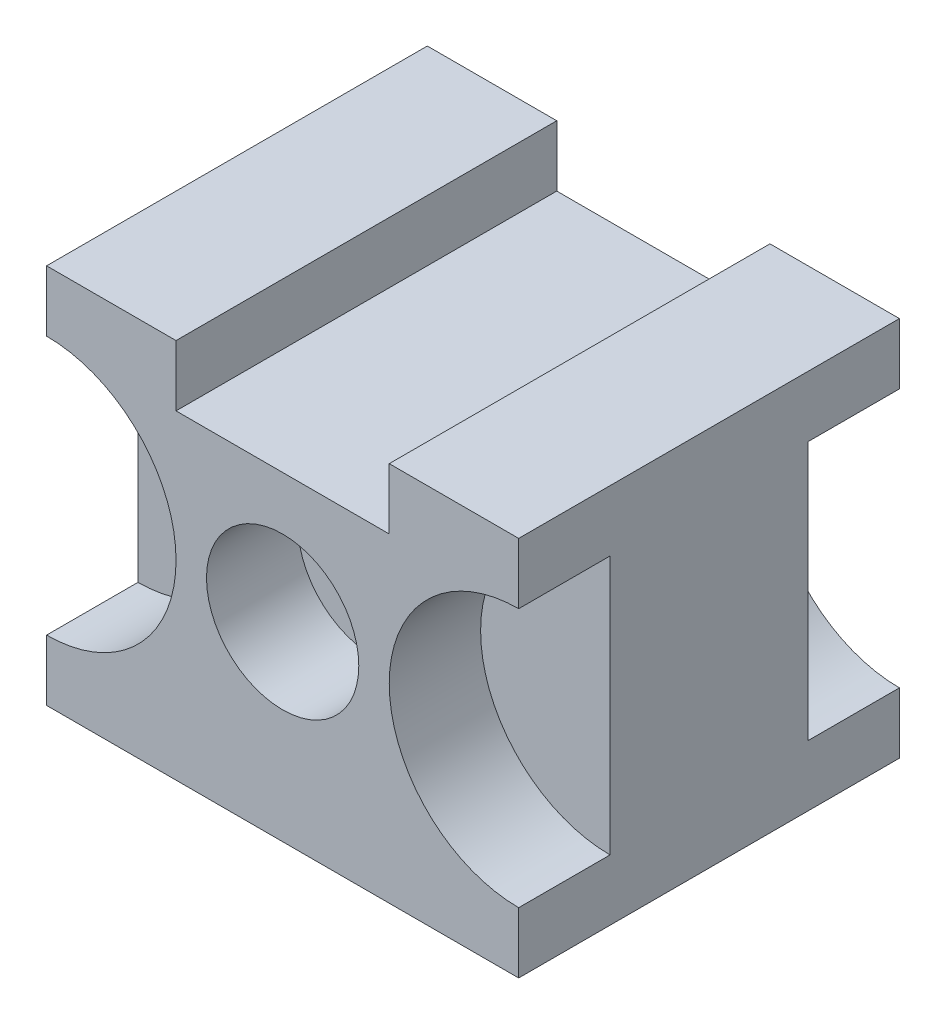
ISO-10303-21;
HEADER;
FILE_DESCRIPTION(('STEP AP214'),'2;1');
FILE_NAME('part.step','',(''),(''),'','','');
FILE_SCHEMA(('AUTOMOTIVE_DESIGN { 1 0 10303 214 1 1 1 1 }'));
ENDSEC;
DATA;
#1=APPLICATION_CONTEXT('core data for automotive mechanical design processes');
#2=APPLICATION_PROTOCOL_DEFINITION('international standard','automotive_design',2000,#1);
#3=PRODUCT_CONTEXT('',#1,'mechanical');
#4=PRODUCT('Part','Part','',(#3));
#5=PRODUCT_RELATED_PRODUCT_CATEGORY('part','',(#4));
#6=PRODUCT_DEFINITION_FORMATION('','',#4);
#7=PRODUCT_DEFINITION_CONTEXT('part definition',#1,'design');
#8=PRODUCT_DEFINITION('design','',#6,#7);
#9=PRODUCT_DEFINITION_SHAPE('','',#8);
#10=(LENGTH_UNIT() NAMED_UNIT(*) SI_UNIT(.MILLI.,.METRE.));
#11=(NAMED_UNIT(*) PLANE_ANGLE_UNIT() SI_UNIT($,.RADIAN.));
#12=(NAMED_UNIT(*) SI_UNIT($,.STERADIAN.) SOLID_ANGLE_UNIT());
#13=UNCERTAINTY_MEASURE_WITH_UNIT(LENGTH_MEASURE(1.E-05),#10,'distance_accuracy_value','');
#14=(GEOMETRIC_REPRESENTATION_CONTEXT(3) GLOBAL_UNCERTAINTY_ASSIGNED_CONTEXT((#13)) GLOBAL_UNIT_ASSIGNED_CONTEXT((#10,
#11,#12)) REPRESENTATION_CONTEXT('',''));
#15=CARTESIAN_POINT('',(0.,0.,0.));
#16=DIRECTION('',(0.,0.,1.));
#17=DIRECTION('',(1.,0.,0.));
#18=AXIS2_PLACEMENT_3D('',#15,#16,#17);
#19=CARTESIAN_POINT('',(62.,50.,50.));
#20=DIRECTION('',(0.,-1.,0.));
#21=DIRECTION('',(1.,0.,0.));
#22=AXIS2_PLACEMENT_3D('',#19,#20,#21);
#23=PLANE('',#22);
#24=DIRECTION('',(-1.,0.,0.));
#25=VECTOR('',#24,1.);
#26=CARTESIAN_POINT('',(62.,50.,50.));
#27=LINE('',#26,#25);
#28=CARTESIAN_POINT('',(17.,50.,50.));
#29=VERTEX_POINT('',#28);
#30=CARTESIAN_POINT('',(0.,50.,50.));
#31=VERTEX_POINT('',#30);
#32=EDGE_CURVE('E286',#29,#31,#27,.T.);
#33=ORIENTED_EDGE('',*,*,#32,.F.);
#34=DIRECTION('',(0.,0.,1.));
#35=VECTOR('',#34,1.);
#36=CARTESIAN_POINT('',(17.,50.,0.));
#37=LINE('',#36,#35);
#38=CARTESIAN_POINT('',(17.,50.,0.));
#39=VERTEX_POINT('',#38);
#40=EDGE_CURVE('E253',#39,#29,#37,.T.);
#41=ORIENTED_EDGE('',*,*,#40,.F.);
#42=DIRECTION('',(-1.,0.,0.));
#43=VECTOR('',#42,1.);
#44=CARTESIAN_POINT('',(62.,50.,0.));
#45=LINE('',#44,#43);
#46=CARTESIAN_POINT('',(0.,50.,0.));
#47=VERTEX_POINT('',#46);
#48=EDGE_CURVE('E299',#39,#47,#45,.T.);
#49=ORIENTED_EDGE('',*,*,#48,.T.);
#50=DIRECTION('',(0.,0.,-1.));
#51=VECTOR('',#50,1.);
#52=CARTESIAN_POINT('',(0.,50.,50.));
#53=LINE('',#52,#51);
#54=EDGE_CURVE('E295',#31,#47,#53,.T.);
#55=ORIENTED_EDGE('',*,*,#54,.F.);
#56=EDGE_LOOP('',(#33,#41,#49,#55));
#57=FACE_BOUND('',#56,.T.);
#58=ADVANCED_FACE('F39',(#57),#23,.F.);
#59=CARTESIAN_POINT('',(0.,50.,50.));
#60=DIRECTION('',(1.,0.,0.));
#61=DIRECTION('',(0.,1.,0.));
#62=AXIS2_PLACEMENT_3D('',#59,#60,#61);
#63=PLANE('',#62);
#64=DIRECTION('',(0.,0.,-1.));
#65=VECTOR('',#64,1.);
#66=CARTESIAN_POINT('',(0.,34.,25.));
#67=LINE('',#66,#65);
#68=CARTESIAN_POINT('',(0.,34.,32.));
#69=VERTEX_POINT('',#68);
#70=CARTESIAN_POINT('',(0.,34.,19.4759366020386));
#71=VERTEX_POINT('',#70);
#72=EDGE_CURVE('E199',#69,#71,#67,.T.);
#73=ORIENTED_EDGE('',*,*,#72,.F.);
#74=DIRECTION('',(0.,1.,0.));
#75=VECTOR('',#74,1.);
#76=CARTESIAN_POINT('',(0.,16.,32.));
#77=LINE('',#76,#75);
#78=CARTESIAN_POINT('',(0.,16.,32.));
#79=VERTEX_POINT('',#78);
#80=EDGE_CURVE('E204',#79,#69,#77,.T.);
#81=ORIENTED_EDGE('',*,*,#80,.F.);
#82=DIRECTION('',(0.,0.,1.));
#83=VECTOR('',#82,1.);
#84=CARTESIAN_POINT('',(0.,16.,19.4759366020386));
#85=LINE('',#84,#83);
#86=CARTESIAN_POINT('',(0.,16.,19.4759366020386));
#87=VERTEX_POINT('',#86);
#88=EDGE_CURVE('E218',#87,#79,#85,.T.);
#89=ORIENTED_EDGE('',*,*,#88,.F.);
#90=DIRECTION('',(0.,-1.,0.));
#91=VECTOR('',#90,1.);
#92=CARTESIAN_POINT('',(0.,34.,19.4759366020386));
#93=LINE('',#92,#91);
#94=EDGE_CURVE('E216',#71,#87,#93,.T.);
#95=ORIENTED_EDGE('',*,*,#94,.F.);
#96=EDGE_LOOP('',(#73,#81,#89,#95));
#97=FACE_BOUND('',#96,.T.);
#98=DIRECTION('',(0.,1.,0.));
#99=VECTOR('',#98,1.);
#100=CARTESIAN_POINT('',(0.,50.,12.));
#101=LINE('',#100,#99);
#102=CARTESIAN_POINT('',(0.,8.,12.));
#103=VERTEX_POINT('',#102);
#104=CARTESIAN_POINT('',(0.,42.,12.));
#105=VERTEX_POINT('',#104);
#106=EDGE_CURVE('E11',#103,#105,#101,.T.);
#107=ORIENTED_EDGE('',*,*,#106,.F.);
#108=DIRECTION('',(0.,0.,-1.));
#109=VECTOR('',#108,1.);
#110=CARTESIAN_POINT('',(0.,8.00000000000001,12.));
#111=LINE('',#110,#109);
#112=CARTESIAN_POINT('',(0.,8.,0.));
#113=VERTEX_POINT('',#112);
#114=EDGE_CURVE('E185',#103,#113,#111,.T.);
#115=ORIENTED_EDGE('',*,*,#114,.T.);
#116=DIRECTION('',(0.,-1.,0.));
#117=VECTOR('',#116,1.);
#118=CARTESIAN_POINT('',(0.,50.,0.));
#119=LINE('',#118,#117);
#120=CARTESIAN_POINT('',(0.,0.,0.));
#121=VERTEX_POINT('',#120);
#122=EDGE_CURVE('E280',#113,#121,#119,.T.);
#123=ORIENTED_EDGE('',*,*,#122,.T.);
#124=DIRECTION('',(0.,0.,-1.));
#125=VECTOR('',#124,1.);
#126=CARTESIAN_POINT('',(0.,0.,50.));
#127=LINE('',#126,#125);
#128=CARTESIAN_POINT('',(0.,0.,50.));
#129=VERTEX_POINT('',#128);
#130=EDGE_CURVE('E313',#129,#121,#127,.T.);
#131=ORIENTED_EDGE('',*,*,#130,.F.);
#132=DIRECTION('',(0.,-1.,0.));
#133=VECTOR('',#132,1.);
#134=CARTESIAN_POINT('',(0.,50.,50.));
#135=LINE('',#134,#133);
#136=CARTESIAN_POINT('',(0.,8.00000000000001,50.));
#137=VERTEX_POINT('',#136);
#138=EDGE_CURVE('E285',#137,#129,#135,.T.);
#139=ORIENTED_EDGE('',*,*,#138,.F.);
#140=DIRECTION('',(0.,0.,1.));
#141=VECTOR('',#140,1.);
#142=CARTESIAN_POINT('',(0.,8.00000000000001,38.));
#143=LINE('',#142,#141);
#144=CARTESIAN_POINT('',(0.,8.,38.));
#145=VERTEX_POINT('',#144);
#146=EDGE_CURVE('E261',#137,#145,#143,.F.);
#147=ORIENTED_EDGE('',*,*,#146,.T.);
#148=DIRECTION('',(0.,-1.,0.));
#149=VECTOR('',#148,1.);
#150=CARTESIAN_POINT('',(0.,50.,38.));
#151=LINE('',#150,#149);
#152=CARTESIAN_POINT('',(0.,42.,38.));
#153=VERTEX_POINT('',#152);
#154=EDGE_CURVE('E318',#153,#145,#151,.T.);
#155=ORIENTED_EDGE('',*,*,#154,.F.);
#156=DIRECTION('',(0.,0.,1.));
#157=VECTOR('',#156,1.);
#158=CARTESIAN_POINT('',(0.,42.,38.));
#159=LINE('',#158,#157);
#160=CARTESIAN_POINT('',(0.,42.,50.));
#161=VERTEX_POINT('',#160);
#162=EDGE_CURVE('E268',#153,#161,#159,.T.);
#163=ORIENTED_EDGE('',*,*,#162,.T.);
#164=EDGE_CURVE('E279',#31,#161,#135,.T.);
#165=ORIENTED_EDGE('',*,*,#164,.F.);
#166=ORIENTED_EDGE('',*,*,#54,.T.);
#167=CARTESIAN_POINT('',(0.,42.,0.));
#168=VERTEX_POINT('',#167);
#169=EDGE_CURVE('E188',#47,#168,#119,.T.);
#170=ORIENTED_EDGE('',*,*,#169,.T.);
#171=DIRECTION('',(0.,0.,-1.));
#172=VECTOR('',#171,1.);
#173=CARTESIAN_POINT('',(0.,42.,12.));
#174=LINE('',#173,#172);
#175=EDGE_CURVE('E53',#168,#105,#174,.F.);
#176=ORIENTED_EDGE('',*,*,#175,.T.);
#177=EDGE_LOOP('',(#107,#115,#123,#131,#139,#147,#155,#163,#165,#166,#170,#176));
#178=FACE_BOUND('',#177,.T.);
#179=ADVANCED_FACE('F41',(#97,#178),#63,.F.);
#180=CARTESIAN_POINT('',(0.,0.,50.));
#181=DIRECTION('',(0.,1.,0.));
#182=DIRECTION('',(0.,0.,1.));
#183=AXIS2_PLACEMENT_3D('',#180,#181,#182);
#184=PLANE('',#183);
#185=DIRECTION('',(1.,0.,0.));
#186=VECTOR('',#185,1.);
#187=CARTESIAN_POINT('',(0.,0.,0.));
#188=LINE('',#187,#186);
#189=CARTESIAN_POINT('',(62.,0.,0.));
#190=VERTEX_POINT('',#189);
#191=EDGE_CURVE('E294',#121,#190,#188,.T.);
#192=ORIENTED_EDGE('',*,*,#191,.T.);
#193=DIRECTION('',(0.,0.,-1.));
#194=VECTOR('',#193,1.);
#195=CARTESIAN_POINT('',(62.,0.,50.));
#196=LINE('',#195,#194);
#197=CARTESIAN_POINT('',(62.,0.,50.));
#198=VERTEX_POINT('',#197);
#199=EDGE_CURVE('E306',#198,#190,#196,.T.);
#200=ORIENTED_EDGE('',*,*,#199,.F.);
#201=DIRECTION('',(1.,0.,0.));
#202=VECTOR('',#201,1.);
#203=CARTESIAN_POINT('',(0.,0.,50.));
#204=LINE('',#203,#202);
#205=EDGE_CURVE('E281',#129,#198,#204,.T.);
#206=ORIENTED_EDGE('',*,*,#205,.F.);
#207=ORIENTED_EDGE('',*,*,#130,.T.);
#208=EDGE_LOOP('',(#192,#200,#206,#207));
#209=FACE_BOUND('',#208,.T.);
#210=ADVANCED_FACE('F376',(#209),#184,.F.);
#211=CARTESIAN_POINT('',(62.,0.,50.));
#212=DIRECTION('',(-1.,0.,0.));
#213=DIRECTION('',(0.,0.,1.));
#214=AXIS2_PLACEMENT_3D('',#211,#212,#213);
#215=PLANE('',#214);
#216=DIRECTION('',(0.,-1.,0.));
#217=VECTOR('',#216,1.);
#218=CARTESIAN_POINT('',(62.,0.,12.));
#219=LINE('',#218,#217);
#220=CARTESIAN_POINT('',(62.,42.,12.));
#221=VERTEX_POINT('',#220);
#222=CARTESIAN_POINT('',(62.,8.,12.));
#223=VERTEX_POINT('',#222);
#224=EDGE_CURVE('E50',#221,#223,#219,.T.);
#225=ORIENTED_EDGE('',*,*,#224,.F.);
#226=DIRECTION('',(0.,0.,-1.));
#227=VECTOR('',#226,1.);
#228=CARTESIAN_POINT('',(62.,42.,12.));
#229=LINE('',#228,#227);
#230=CARTESIAN_POINT('',(62.,42.,0.));
#231=VERTEX_POINT('',#230);
#232=EDGE_CURVE('E197',#221,#231,#229,.T.);
#233=ORIENTED_EDGE('',*,*,#232,.T.);
#234=DIRECTION('',(0.,1.,0.));
#235=VECTOR('',#234,1.);
#236=CARTESIAN_POINT('',(62.,0.,0.));
#237=LINE('',#236,#235);
#238=CARTESIAN_POINT('',(62.,50.,0.));
#239=VERTEX_POINT('',#238);
#240=EDGE_CURVE('E296',#231,#239,#237,.T.);
#241=ORIENTED_EDGE('',*,*,#240,.T.);
#242=DIRECTION('',(0.,0.,-1.));
#243=VECTOR('',#242,1.);
#244=CARTESIAN_POINT('',(62.,50.,50.));
#245=LINE('',#244,#243);
#246=CARTESIAN_POINT('',(62.,50.,50.));
#247=VERTEX_POINT('',#246);
#248=EDGE_CURVE('E304',#247,#239,#245,.T.);
#249=ORIENTED_EDGE('',*,*,#248,.F.);
#250=DIRECTION('',(0.,1.,0.));
#251=VECTOR('',#250,1.);
#252=CARTESIAN_POINT('',(62.,0.,50.));
#253=LINE('',#252,#251);
#254=CARTESIAN_POINT('',(62.,42.,50.));
#255=VERTEX_POINT('',#254);
#256=EDGE_CURVE('E283',#255,#247,#253,.T.);
#257=ORIENTED_EDGE('',*,*,#256,.F.);
#258=DIRECTION('',(0.,0.,1.));
#259=VECTOR('',#258,1.);
#260=CARTESIAN_POINT('',(62.,42.,38.));
#261=LINE('',#260,#259);
#262=CARTESIAN_POINT('',(62.,42.,38.));
#263=VERTEX_POINT('',#262);
#264=EDGE_CURVE('E271',#255,#263,#261,.F.);
#265=ORIENTED_EDGE('',*,*,#264,.T.);
#266=DIRECTION('',(0.,1.,0.));
#267=VECTOR('',#266,1.);
#268=CARTESIAN_POINT('',(62.,0.,38.));
#269=LINE('',#268,#267);
#270=CARTESIAN_POINT('',(62.,8.00000000000001,38.));
#271=VERTEX_POINT('',#270);
#272=EDGE_CURVE('E316',#271,#263,#269,.T.);
#273=ORIENTED_EDGE('',*,*,#272,.F.);
#274=DIRECTION('',(0.,0.,1.));
#275=VECTOR('',#274,1.);
#276=CARTESIAN_POINT('',(62.,8.00000000000001,38.));
#277=LINE('',#276,#275);
#278=CARTESIAN_POINT('',(62.,8.00000000000001,50.));
#279=VERTEX_POINT('',#278);
#280=EDGE_CURVE('E273',#271,#279,#277,.T.);
#281=ORIENTED_EDGE('',*,*,#280,.T.);
#282=EDGE_CURVE('E284',#198,#279,#253,.T.);
#283=ORIENTED_EDGE('',*,*,#282,.F.);
#284=ORIENTED_EDGE('',*,*,#199,.T.);
#285=CARTESIAN_POINT('',(62.,8.,0.));
#286=VERTEX_POINT('',#285);
#287=EDGE_CURVE('E300',#190,#286,#237,.T.);
#288=ORIENTED_EDGE('',*,*,#287,.T.);
#289=DIRECTION('',(0.,0.,-1.));
#290=VECTOR('',#289,1.);
#291=CARTESIAN_POINT('',(62.,8.,12.));
#292=LINE('',#291,#290);
#293=EDGE_CURVE('E65',#286,#223,#292,.F.);
#294=ORIENTED_EDGE('',*,*,#293,.T.);
#295=EDGE_LOOP('',(#225,#233,#241,#249,#257,#265,#273,#281,#283,#284,#288,#294));
#296=FACE_BOUND('',#295,.T.);
#297=ADVANCED_FACE('F326',(#296),#215,.F.);
#298=CARTESIAN_POINT('',(45.,50.,0.));
#299=VERTEX_POINT('',#298);
#300=EDGE_CURVE('E303',#239,#299,#45,.T.);
#301=ORIENTED_EDGE('',*,*,#300,.T.);
#302=DIRECTION('',(0.,0.,1.));
#303=VECTOR('',#302,1.);
#304=CARTESIAN_POINT('',(45.,50.,0.));
#305=LINE('',#304,#303);
#306=CARTESIAN_POINT('',(45.,50.,50.));
#307=VERTEX_POINT('',#306);
#308=EDGE_CURVE('E251',#299,#307,#305,.T.);
#309=ORIENTED_EDGE('',*,*,#308,.T.);
#310=EDGE_CURVE('E287',#247,#307,#27,.T.);
#311=ORIENTED_EDGE('',*,*,#310,.F.);
#312=ORIENTED_EDGE('',*,*,#248,.T.);
#313=EDGE_LOOP('',(#301,#309,#311,#312));
#314=FACE_BOUND('',#313,.T.);
#315=ADVANCED_FACE('F339',(#314),#23,.F.);
#316=CARTESIAN_POINT('',(0.,0.,50.));
#317=DIRECTION('',(0.,0.,1.));
#318=DIRECTION('',(1.,0.,0.));
#319=AXIS2_PLACEMENT_3D('',#316,#317,#318);
#320=PLANE('',#319);
#321=CARTESIAN_POINT('',(31.,25.,50.));
#322=DIRECTION('',(0.,0.,1.));
#323=DIRECTION('',(1.,0.,0.));
#324=AXIS2_PLACEMENT_3D('',#321,#322,#323);
#325=CIRCLE('',#324,10.);
#326=CARTESIAN_POINT('',(41.,25.,50.));
#327=VERTEX_POINT('',#326);
#328=EDGE_CURVE('E405',#327,#327,#325,.T.);
#329=ORIENTED_EDGE('',*,*,#328,.F.);
#330=EDGE_LOOP('',(#329));
#331=FACE_BOUND('',#330,.T.);
#332=DIRECTION('',(0.,-1.,0.));
#333=VECTOR('',#332,1.);
#334=CARTESIAN_POINT('',(17.,42.,50.));
#335=LINE('',#334,#333);
#336=CARTESIAN_POINT('',(17.,42.,50.));
#337=VERTEX_POINT('',#336);
#338=EDGE_CURVE('E243',#29,#337,#335,.T.);
#339=ORIENTED_EDGE('',*,*,#338,.F.);
#340=ORIENTED_EDGE('',*,*,#32,.T.);
#341=ORIENTED_EDGE('',*,*,#164,.T.);
#342=CARTESIAN_POINT('',(0.,25.,50.));
#343=DIRECTION('',(0.,0.,1.));
#344=DIRECTION('',(1.,0.,0.));
#345=AXIS2_PLACEMENT_3D('',#342,#343,#344);
#346=CIRCLE('',#345,17.);
#347=EDGE_CURVE('E314',#137,#161,#346,.T.);
#348=ORIENTED_EDGE('',*,*,#347,.F.);
#349=ORIENTED_EDGE('',*,*,#138,.T.);
#350=ORIENTED_EDGE('',*,*,#205,.T.);
#351=ORIENTED_EDGE('',*,*,#282,.T.);
#352=CARTESIAN_POINT('',(62.,25.,50.));
#353=DIRECTION('',(0.,0.,1.));
#354=DIRECTION('',(1.,0.,0.));
#355=AXIS2_PLACEMENT_3D('',#352,#353,#354);
#356=CIRCLE('',#355,17.);
#357=EDGE_CURVE('E265',#255,#279,#356,.T.);
#358=ORIENTED_EDGE('',*,*,#357,.F.);
#359=ORIENTED_EDGE('',*,*,#256,.T.);
#360=ORIENTED_EDGE('',*,*,#310,.T.);
#361=DIRECTION('',(0.,1.,0.));
#362=VECTOR('',#361,1.);
#363=CARTESIAN_POINT('',(45.,50.,50.));
#364=LINE('',#363,#362);
#365=CARTESIAN_POINT('',(45.,42.,50.));
#366=VERTEX_POINT('',#365);
#367=EDGE_CURVE('E226',#366,#307,#364,.T.);
#368=ORIENTED_EDGE('',*,*,#367,.F.);
#369=DIRECTION('',(1.,0.,0.));
#370=VECTOR('',#369,1.);
#371=CARTESIAN_POINT('',(31.,42.,50.));
#372=LINE('',#371,#370);
#373=EDGE_CURVE('E237',#337,#366,#372,.T.);
#374=ORIENTED_EDGE('',*,*,#373,.F.);
#375=EDGE_LOOP('',(#339,#340,#341,#348,#349,#350,#351,#358,#359,#360,#368,#374));
#376=FACE_BOUND('',#375,.T.);
#377=ADVANCED_FACE('F350',(#331,#376),#320,.T.);
#378=CARTESIAN_POINT('',(0.,0.,0.));
#379=DIRECTION('',(0.,0.,1.));
#380=DIRECTION('',(1.,0.,0.));
#381=AXIS2_PLACEMENT_3D('',#378,#379,#380);
#382=PLANE('',#381);
#383=ORIENTED_EDGE('',*,*,#240,.F.);
#384=CARTESIAN_POINT('',(62.,25.,0.));
#385=DIRECTION('',(0.,0.,1.));
#386=DIRECTION('',(1.,0.,0.));
#387=AXIS2_PLACEMENT_3D('',#384,#385,#386);
#388=CIRCLE('',#387,17.);
#389=EDGE_CURVE('E319',#231,#286,#388,.T.);
#390=ORIENTED_EDGE('',*,*,#389,.T.);
#391=ORIENTED_EDGE('',*,*,#287,.F.);
#392=ORIENTED_EDGE('',*,*,#191,.F.);
#393=ORIENTED_EDGE('',*,*,#122,.F.);
#394=CARTESIAN_POINT('',(0.,25.,0.));
#395=DIRECTION('',(0.,0.,-1.));
#396=DIRECTION('',(-1.,0.,0.));
#397=AXIS2_PLACEMENT_3D('',#394,#395,#396);
#398=CIRCLE('',#397,17.);
#399=EDGE_CURVE('E184',#168,#113,#398,.T.);
#400=ORIENTED_EDGE('',*,*,#399,.F.);
#401=ORIENTED_EDGE('',*,*,#169,.F.);
#402=ORIENTED_EDGE('',*,*,#48,.F.);
#403=DIRECTION('',(0.,-1.,0.));
#404=VECTOR('',#403,1.);
#405=CARTESIAN_POINT('',(17.,42.,0.));
#406=LINE('',#405,#404);
#407=CARTESIAN_POINT('',(17.,42.,0.));
#408=VERTEX_POINT('',#407);
#409=EDGE_CURVE('E239',#39,#408,#406,.T.);
#410=ORIENTED_EDGE('',*,*,#409,.T.);
#411=DIRECTION('',(1.,0.,0.));
#412=VECTOR('',#411,1.);
#413=CARTESIAN_POINT('',(45.,42.,0.));
#414=LINE('',#413,#412);
#415=CARTESIAN_POINT('',(45.,42.,0.));
#416=VERTEX_POINT('',#415);
#417=EDGE_CURVE('E235',#408,#416,#414,.T.);
#418=ORIENTED_EDGE('',*,*,#417,.T.);
#419=DIRECTION('',(0.,1.,0.));
#420=VECTOR('',#419,1.);
#421=CARTESIAN_POINT('',(45.,50.,0.));
#422=LINE('',#421,#420);
#423=EDGE_CURVE('E234',#416,#299,#422,.T.);
#424=ORIENTED_EDGE('',*,*,#423,.T.);
#425=ORIENTED_EDGE('',*,*,#300,.F.);
#426=EDGE_LOOP('',(#383,#390,#391,#392,#393,#400,#401,#402,#410,#418,#424,#425));
#427=FACE_BOUND('',#426,.T.);
#428=ADVANCED_FACE('F334',(#427),#382,.F.);
#429=CARTESIAN_POINT('',(0.,25.,38.));
#430=DIRECTION('',(0.,0.,1.));
#431=DIRECTION('',(1.,0.,0.));
#432=AXIS2_PLACEMENT_3D('',#429,#430,#431);
#433=PLANE('',#432);
#434=ORIENTED_EDGE('',*,*,#154,.T.);
#435=CARTESIAN_POINT('',(0.,25.,38.));
#436=DIRECTION('',(0.,0.,1.));
#437=DIRECTION('',(1.,0.,0.));
#438=AXIS2_PLACEMENT_3D('',#435,#436,#437);
#439=CIRCLE('',#438,17.);
#440=EDGE_CURVE('E249',#145,#153,#439,.T.);
#441=ORIENTED_EDGE('',*,*,#440,.T.);
#442=EDGE_LOOP('',(#434,#441));
#443=FACE_BOUND('',#442,.T.);
#444=ADVANCED_FACE('F364',(#443),#433,.T.);
#445=CARTESIAN_POINT('',(0.,25.,38.));
#446=DIRECTION('',(0.,0.,1.));
#447=DIRECTION('',(1.,0.,0.));
#448=AXIS2_PLACEMENT_3D('',#445,#446,#447);
#449=CYLINDRICAL_SURFACE('',#448,17.);
#450=ORIENTED_EDGE('',*,*,#440,.F.);
#451=ORIENTED_EDGE('',*,*,#146,.F.);
#452=ORIENTED_EDGE('',*,*,#347,.T.);
#453=ORIENTED_EDGE('',*,*,#162,.F.);
#454=EDGE_LOOP('',(#450,#451,#452,#453));
#455=FACE_BOUND('',#454,.T.);
#456=ADVANCED_FACE('F360',(#455),#449,.F.);
#457=CARTESIAN_POINT('',(62.,25.,38.));
#458=DIRECTION('',(0.,0.,1.));
#459=DIRECTION('',(1.,0.,0.));
#460=AXIS2_PLACEMENT_3D('',#457,#458,#459);
#461=PLANE('',#460);
#462=ORIENTED_EDGE('',*,*,#272,.T.);
#463=CARTESIAN_POINT('',(62.,25.,38.));
#464=DIRECTION('',(0.,0.,1.));
#465=DIRECTION('',(1.,0.,0.));
#466=AXIS2_PLACEMENT_3D('',#463,#464,#465);
#467=CIRCLE('',#466,17.);
#468=EDGE_CURVE('E256',#263,#271,#467,.T.);
#469=ORIENTED_EDGE('',*,*,#468,.T.);
#470=EDGE_LOOP('',(#462,#469));
#471=FACE_BOUND('',#470,.T.);
#472=ADVANCED_FACE('F354',(#471),#461,.T.);
#473=CARTESIAN_POINT('',(62.,25.,38.));
#474=DIRECTION('',(0.,0.,1.));
#475=DIRECTION('',(1.,0.,0.));
#476=AXIS2_PLACEMENT_3D('',#473,#474,#475);
#477=CYLINDRICAL_SURFACE('',#476,17.);
#478=ORIENTED_EDGE('',*,*,#468,.F.);
#479=ORIENTED_EDGE('',*,*,#264,.F.);
#480=ORIENTED_EDGE('',*,*,#357,.T.);
#481=ORIENTED_EDGE('',*,*,#280,.F.);
#482=EDGE_LOOP('',(#478,#479,#480,#481));
#483=FACE_BOUND('',#482,.T.);
#484=ADVANCED_FACE('F352',(#483),#477,.F.);
#485=CARTESIAN_POINT('',(31.,42.,0.));
#486=DIRECTION('',(0.,-1.,0.));
#487=DIRECTION('',(1.,0.,0.));
#488=AXIS2_PLACEMENT_3D('',#485,#486,#487);
#489=PLANE('',#488);
#490=ORIENTED_EDGE('',*,*,#373,.T.);
#491=DIRECTION('',(0.,0.,1.));
#492=VECTOR('',#491,1.);
#493=CARTESIAN_POINT('',(45.,42.,0.));
#494=LINE('',#493,#492);
#495=EDGE_CURVE('E245',#416,#366,#494,.T.);
#496=ORIENTED_EDGE('',*,*,#495,.F.);
#497=ORIENTED_EDGE('',*,*,#417,.F.);
#498=DIRECTION('',(0.,0.,1.));
#499=VECTOR('',#498,1.);
#500=CARTESIAN_POINT('',(17.,42.,0.));
#501=LINE('',#500,#499);
#502=EDGE_CURVE('E246',#408,#337,#501,.T.);
#503=ORIENTED_EDGE('',*,*,#502,.T.);
#504=EDGE_LOOP('',(#490,#496,#497,#503));
#505=FACE_BOUND('',#504,.T.);
#506=ADVANCED_FACE('F361',(#505),#489,.F.);
#507=CARTESIAN_POINT('',(17.,42.,0.));
#508=DIRECTION('',(-1.,0.,0.));
#509=DIRECTION('',(0.,0.,1.));
#510=AXIS2_PLACEMENT_3D('',#507,#508,#509);
#511=PLANE('',#510);
#512=ORIENTED_EDGE('',*,*,#338,.T.);
#513=ORIENTED_EDGE('',*,*,#502,.F.);
#514=ORIENTED_EDGE('',*,*,#409,.F.);
#515=ORIENTED_EDGE('',*,*,#40,.T.);
#516=EDGE_LOOP('',(#512,#513,#514,#515));
#517=FACE_BOUND('',#516,.T.);
#518=ADVANCED_FACE('F448',(#517),#511,.F.);
#519=CARTESIAN_POINT('',(45.,50.,0.));
#520=DIRECTION('',(1.,0.,0.));
#521=DIRECTION('',(0.,0.,-1.));
#522=AXIS2_PLACEMENT_3D('',#519,#520,#521);
#523=PLANE('',#522);
#524=ORIENTED_EDGE('',*,*,#367,.T.);
#525=ORIENTED_EDGE('',*,*,#308,.F.);
#526=ORIENTED_EDGE('',*,*,#423,.F.);
#527=ORIENTED_EDGE('',*,*,#495,.T.);
#528=EDGE_LOOP('',(#524,#525,#526,#527));
#529=FACE_BOUND('',#528,.T.);
#530=ADVANCED_FACE('F341',(#529),#523,.F.);
#531=CARTESIAN_POINT('',(12.,16.,32.));
#532=DIRECTION('',(0.,0.,1.));
#533=DIRECTION('',(0.,-1.,0.));
#534=AXIS2_PLACEMENT_3D('',#531,#532,#533);
#535=PLANE('',#534);
#536=ORIENTED_EDGE('',*,*,#80,.T.);
#537=DIRECTION('',(-1.,0.,0.));
#538=VECTOR('',#537,1.);
#539=CARTESIAN_POINT('',(12.,34.,32.));
#540=LINE('',#539,#538);
#541=CARTESIAN_POINT('',(12.,34.,32.));
#542=VERTEX_POINT('',#541);
#543=EDGE_CURVE('E224',#542,#69,#540,.T.);
#544=ORIENTED_EDGE('',*,*,#543,.F.);
#545=DIRECTION('',(0.,1.,0.));
#546=VECTOR('',#545,1.);
#547=CARTESIAN_POINT('',(12.,16.,32.));
#548=LINE('',#547,#546);
#549=CARTESIAN_POINT('',(12.,16.,32.));
#550=VERTEX_POINT('',#549);
#551=EDGE_CURVE('E209',#550,#542,#548,.T.);
#552=ORIENTED_EDGE('',*,*,#551,.F.);
#553=DIRECTION('',(-1.,0.,0.));
#554=VECTOR('',#553,1.);
#555=CARTESIAN_POINT('',(12.,16.,32.));
#556=LINE('',#555,#554);
#557=EDGE_CURVE('E230',#550,#79,#556,.T.);
#558=ORIENTED_EDGE('',*,*,#557,.T.);
#559=EDGE_LOOP('',(#536,#544,#552,#558));
#560=FACE_BOUND('',#559,.T.);
#561=ADVANCED_FACE('F433',(#560),#535,.F.);
#562=CARTESIAN_POINT('',(12.,16.,19.4759366020386));
#563=DIRECTION('',(0.,-1.,0.));
#564=DIRECTION('',(1.,0.,0.));
#565=AXIS2_PLACEMENT_3D('',#562,#563,#564);
#566=PLANE('',#565);
#567=ORIENTED_EDGE('',*,*,#88,.T.);
#568=ORIENTED_EDGE('',*,*,#557,.F.);
#569=DIRECTION('',(0.,0.,1.));
#570=VECTOR('',#569,1.);
#571=CARTESIAN_POINT('',(12.,16.,19.4759366020386));
#572=LINE('',#571,#570);
#573=CARTESIAN_POINT('',(12.,16.,19.4759366020386));
#574=VERTEX_POINT('',#573);
#575=EDGE_CURVE('E210',#574,#550,#572,.T.);
#576=ORIENTED_EDGE('',*,*,#575,.F.);
#577=DIRECTION('',(-1.,0.,0.));
#578=VECTOR('',#577,1.);
#579=CARTESIAN_POINT('',(12.,16.,19.4759366020386));
#580=LINE('',#579,#578);
#581=EDGE_CURVE('E228',#574,#87,#580,.T.);
#582=ORIENTED_EDGE('',*,*,#581,.T.);
#583=EDGE_LOOP('',(#567,#568,#576,#582));
#584=FACE_BOUND('',#583,.T.);
#585=ADVANCED_FACE('F436',(#584),#566,.F.);
#586=CARTESIAN_POINT('',(12.,34.,19.4759366020386));
#587=DIRECTION('',(0.,0.,-1.));
#588=DIRECTION('',(0.,1.,0.));
#589=AXIS2_PLACEMENT_3D('',#586,#587,#588);
#590=PLANE('',#589);
#591=ORIENTED_EDGE('',*,*,#94,.T.);
#592=ORIENTED_EDGE('',*,*,#581,.F.);
#593=DIRECTION('',(0.,-1.,0.));
#594=VECTOR('',#593,1.);
#595=CARTESIAN_POINT('',(12.,34.,19.4759366020386));
#596=LINE('',#595,#594);
#597=CARTESIAN_POINT('',(12.,34.,19.4759366020386));
#598=VERTEX_POINT('',#597);
#599=EDGE_CURVE('E201',#598,#574,#596,.T.);
#600=ORIENTED_EDGE('',*,*,#599,.F.);
#601=DIRECTION('',(-1.,0.,0.));
#602=VECTOR('',#601,1.);
#603=CARTESIAN_POINT('',(12.,34.,19.4759366020386));
#604=LINE('',#603,#602);
#605=EDGE_CURVE('E213',#598,#71,#604,.T.);
#606=ORIENTED_EDGE('',*,*,#605,.T.);
#607=EDGE_LOOP('',(#591,#592,#600,#606));
#608=FACE_BOUND('',#607,.T.);
#609=ADVANCED_FACE('F439',(#608),#590,.F.);
#610=CARTESIAN_POINT('',(12.,34.,25.));
#611=DIRECTION('',(0.,1.,0.));
#612=DIRECTION('',(-1.,0.,0.));
#613=AXIS2_PLACEMENT_3D('',#610,#611,#612);
#614=PLANE('',#613);
#615=ORIENTED_EDGE('',*,*,#72,.T.);
#616=ORIENTED_EDGE('',*,*,#605,.F.);
#617=DIRECTION('',(0.,0.,-1.));
#618=VECTOR('',#617,1.);
#619=CARTESIAN_POINT('',(12.,34.,32.));
#620=LINE('',#619,#618);
#621=EDGE_CURVE('E203',#542,#598,#620,.T.);
#622=ORIENTED_EDGE('',*,*,#621,.F.);
#623=ORIENTED_EDGE('',*,*,#543,.T.);
#624=EDGE_LOOP('',(#615,#616,#622,#623));
#625=FACE_BOUND('',#624,.T.);
#626=ADVANCED_FACE('F431',(#625),#614,.F.);
#627=CARTESIAN_POINT('',(12.,0.,0.));
#628=DIRECTION('',(-1.,0.,0.));
#629=DIRECTION('',(0.,-1.,0.));
#630=AXIS2_PLACEMENT_3D('',#627,#628,#629);
#631=PLANE('',#630);
#632=ORIENTED_EDGE('',*,*,#621,.T.);
#633=ORIENTED_EDGE('',*,*,#599,.T.);
#634=ORIENTED_EDGE('',*,*,#575,.T.);
#635=ORIENTED_EDGE('',*,*,#551,.T.);
#636=EDGE_LOOP('',(#632,#633,#634,#635));
#637=FACE_BOUND('',#636,.T.);
#638=ADVANCED_FACE('F426',(#637),#631,.T.);
#639=CARTESIAN_POINT('',(0.,25.,12.));
#640=DIRECTION('',(0.,0.,-1.));
#641=DIRECTION('',(-1.,0.,0.));
#642=AXIS2_PLACEMENT_3D('',#639,#640,#641);
#643=PLANE('',#642);
#644=ORIENTED_EDGE('',*,*,#106,.T.);
#645=CARTESIAN_POINT('',(0.,25.,12.));
#646=DIRECTION('',(0.,0.,-1.));
#647=DIRECTION('',(-1.,0.,0.));
#648=AXIS2_PLACEMENT_3D('',#645,#646,#647);
#649=CIRCLE('',#648,17.);
#650=EDGE_CURVE('E176',#105,#103,#649,.T.);
#651=ORIENTED_EDGE('',*,*,#650,.T.);
#652=EDGE_LOOP('',(#644,#651));
#653=FACE_BOUND('',#652,.T.);
#654=ADVANCED_FACE('F180',(#653),#643,.T.);
#655=CARTESIAN_POINT('',(0.,25.,12.));
#656=DIRECTION('',(0.,0.,-1.));
#657=DIRECTION('',(-1.,0.,0.));
#658=AXIS2_PLACEMENT_3D('',#655,#656,#657);
#659=CYLINDRICAL_SURFACE('',#658,17.);
#660=ORIENTED_EDGE('',*,*,#650,.F.);
#661=ORIENTED_EDGE('',*,*,#175,.F.);
#662=ORIENTED_EDGE('',*,*,#399,.T.);
#663=ORIENTED_EDGE('',*,*,#114,.F.);
#664=EDGE_LOOP('',(#660,#661,#662,#663));
#665=FACE_BOUND('',#664,.T.);
#666=ADVANCED_FACE('F182',(#665),#659,.F.);
#667=CARTESIAN_POINT('',(62.,25.,12.));
#668=DIRECTION('',(0.,0.,-1.));
#669=DIRECTION('',(-1.,0.,0.));
#670=AXIS2_PLACEMENT_3D('',#667,#668,#669);
#671=PLANE('',#670);
#672=ORIENTED_EDGE('',*,*,#224,.T.);
#673=CARTESIAN_POINT('',(62.,25.,12.));
#674=DIRECTION('',(0.,0.,-1.));
#675=DIRECTION('',(-1.,0.,0.));
#676=AXIS2_PLACEMENT_3D('',#673,#674,#675);
#677=CIRCLE('',#676,17.);
#678=EDGE_CURVE('E181',#223,#221,#677,.T.);
#679=ORIENTED_EDGE('',*,*,#678,.T.);
#680=EDGE_LOOP('',(#672,#679));
#681=FACE_BOUND('',#680,.T.);
#682=ADVANCED_FACE('F323',(#681),#671,.T.);
#683=CARTESIAN_POINT('',(62.,25.,12.));
#684=DIRECTION('',(0.,0.,-1.));
#685=DIRECTION('',(-1.,0.,0.));
#686=AXIS2_PLACEMENT_3D('',#683,#684,#685);
#687=CYLINDRICAL_SURFACE('',#686,17.);
#688=ORIENTED_EDGE('',*,*,#678,.F.);
#689=ORIENTED_EDGE('',*,*,#293,.F.);
#690=ORIENTED_EDGE('',*,*,#389,.F.);
#691=ORIENTED_EDGE('',*,*,#232,.F.);
#692=EDGE_LOOP('',(#688,#689,#690,#691));
#693=FACE_BOUND('',#692,.T.);
#694=ADVANCED_FACE('F324',(#693),#687,.F.);
#695=CARTESIAN_POINT('',(31.,25.,38.));
#696=DIRECTION('',(0.,0.,1.));
#697=DIRECTION('',(1.,0.,0.));
#698=AXIS2_PLACEMENT_3D('',#695,#696,#697);
#699=CYLINDRICAL_SURFACE('',#698,10.);
#700=CARTESIAN_POINT('',(31.,25.,38.));
#701=DIRECTION('',(0.,0.,1.));
#702=DIRECTION('',(1.,0.,0.));
#703=AXIS2_PLACEMENT_3D('',#700,#701,#702);
#704=CIRCLE('',#703,10.);
#705=CARTESIAN_POINT('',(41.,25.,38.));
#706=VERTEX_POINT('',#705);
#707=EDGE_CURVE('E399',#706,#706,#704,.T.);
#708=ORIENTED_EDGE('',*,*,#707,.F.);
#709=EDGE_LOOP('',(#708));
#710=FACE_BOUND('',#709,.T.);
#711=ORIENTED_EDGE('',*,*,#328,.T.);
#712=EDGE_LOOP('',(#711));
#713=FACE_BOUND('',#712,.T.);
#714=ADVANCED_FACE('F409',(#710,#713),#699,.F.);
#715=CARTESIAN_POINT('',(31.,25.,38.));
#716=DIRECTION('',(0.,0.,1.));
#717=DIRECTION('',(1.,0.,0.));
#718=AXIS2_PLACEMENT_3D('',#715,#716,#717);
#719=PLANE('',#718);
#720=ORIENTED_EDGE('',*,*,#707,.T.);
#721=EDGE_LOOP('',(#720));
#722=FACE_BOUND('',#721,.T.);
#723=ADVANCED_FACE('F415',(#722),#719,.T.);
#724=CLOSED_SHELL('',(#58,#179,#210,#297,#315,#377,#428,#444,#456,#472,#484,#506,#518,#530,#561,
#585,#609,#626,#638,#654,#666,#682,#694,#714,#723));
#725=MANIFOLD_SOLID_BREP('B2',#724);
#726=ADVANCED_BREP_SHAPE_REPRESENTATION('',(#18,#725),#14);
#727=SHAPE_DEFINITION_REPRESENTATION(#9,#726);
ENDSEC;
END-ISO-10303-21;
